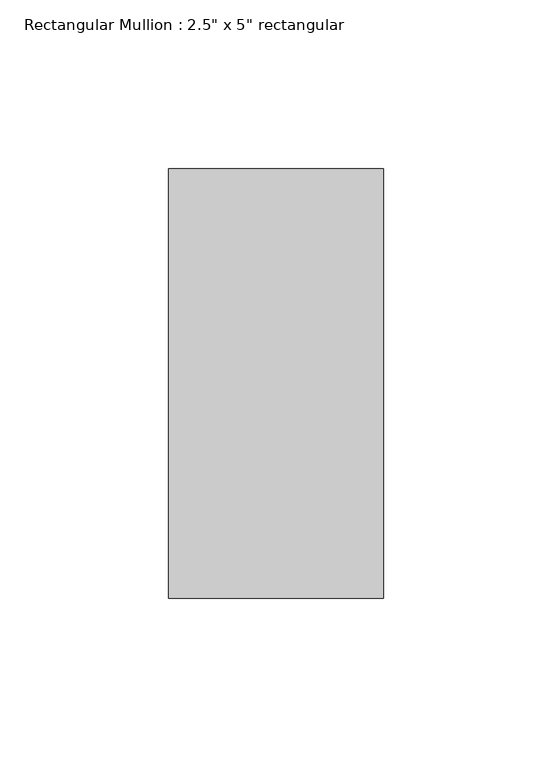
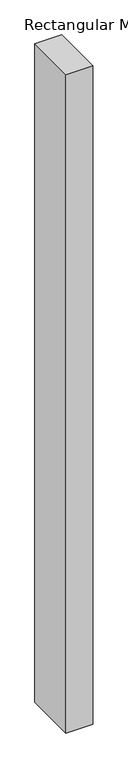
"""IFC4 building model written with IfcOpenShell, lengths in millimetres: member geometry."""

from ifc_helpers import new_model, si_unit, frame, origin, place, context, project, spatial, polyline, outline, extrude, source, transform, mapped, element, save


def member_00baf460(model_context):
    return source(origin(), model_context, "Body", "SweptSolid", [
        extrude(outline(polyline([(0.0, 63.5), (0.0, -63.5), (-63.5, -63.5), (-63.5, 63.5), (0.0, 63.5)])), frame((0.0, 0.0, -1643.8504197), z_axis=(0.0, 0.0, 1.0), x_axis=(1.0, 0.0, 0.0)), (0.0, 0.0, 1.0), 1643.8504197),
    ])


if __name__ == "__main__":
    model = new_model("IFC4")
    model_context = context("Model", 3, world=origin())
    ifc_project = project(units=[si_unit("LENGTHUNIT", "METRE", prefix="MILLI")], contexts=[model_context])
    site = spatial("IfcSite", under=ifc_project)
    building = spatial("IfcBuilding", under=site)
    placement = place(None, origin())
    member_shape = member_00baf460(model_context)
    element("IfcMember", 1, ObjectType="Rectangular Mullion : 2.5\" x 5\" rectangular", at=placement, inside=building, context=model_context, shape_type="MappedRepresentation", body=[
        mapped(member_shape, transform((0.0, 0.0, 0.0), x_axis=(1.0, 0.0, 0.0), y_axis=(0.0, 1.0, 0.0), z_axis=(0.0, 0.0, 1.0))),
    ])
    save(model, "model.ifc")

# Revit data of these elements
# Type "Rectangular Mullion : 2.5\" x 5\" rectangular"
#   built-in parameter 1007304 = 0.416667 (stored number, unit not read)
#   built-in parameter 1007301 = 0.104167 (stored number, unit not read)
#   built-in parameter 1007300 = 0.104167 (stored number, unit not read)
# Element 1 (IfcMember, "Rectangular Mullion : 2.5\" x 5\" rectangular")
#   Materials on its faces: "Aluminum"
# Materials
#   "Aluminum": class "Metal", colour RGB 247 247 247, transparency 0, Description = "Aluminum 6061", Cost = 0
